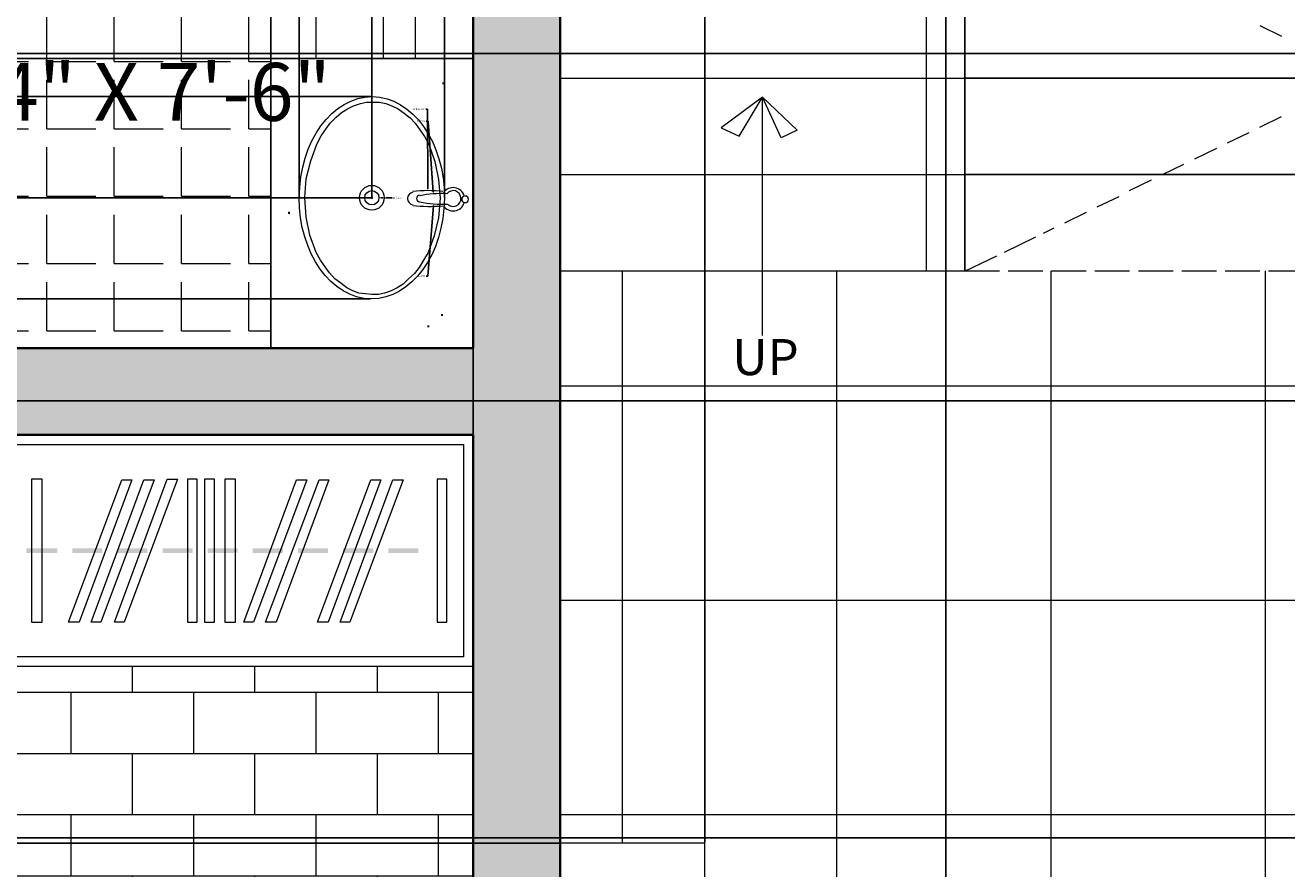
# Model space of a CAD drawing. Units: inches. Extents: x 6 to 575, y 34 to 566.
# Tile 10 of 21: x 151 to 282, y 387 to 474. Entities that reach past the tile are written whole.
import ezdxf

# ---------------------------------------------------------------- set-up
doc = ezdxf.new("R2010")
doc.units = ezdxf.units.IN
doc.linetypes.add('ACAD_ISO02W100', pattern=[15, 12, -3])
for name, color, linetype, lineweight in [('A-ANNO-DIMS', 2, 'Continuous', 18), ('A-ANNO-SYMB', 6, 'Continuous', 18), ('A-ANNO-TEXT', 6, 'Continuous', 18), ('A-AREA-IDEN', 6, 'Continuous', 20), ('A-FLOR-CASE', 2, 'Continuous', 18), ('A-FLOR-FIXT', 9, 'Continuous', 18), ('A-FLOR-PATT', 252, 'Continuous', 9), ('A-FLOR-STRS-OVHD', 1, 'ACAD_ISO02W100', 13), ('A-WALL-PATT', 251, 'Continuous', 9), ('STAIRS', 1, 'Continuous', 20), ('WALLS', 7, 'Continuous', 35)]:
    doc.layers.add(name, color=color, linetype=linetype, lineweight=lineweight)
doc.styles.add('PDF Arial Narrow', font='txt')
doc.styles.add('PDF Century Gothic', font='txt')
doc.styles.get("Standard").update_dxf_attribs({"font": 'arial.ttf'})
doc.dimstyles.get("Standard").update_dxf_attribs({"dimtxt": 0.18, "dimasz": 0.18, "dimexe": 0.18, "dimexo": 0.0625, "dimgap": 0.09, "dimtad": 0, "dimtih": 1, "dimtoh": 1, "dimdec": 4, "dimzin": 0, "dimdsep": 46, "dimtxsty": 'Standard', "dimcen": 0.09, "dimadec": 0, "dimazin": 0, "dimtfac": 1, "dimtdec": 4, "dimtofl": 0, "dimtmove": 0, "dimatfit": 3, "dimfxl": 1, "dimtolj": 1, "dimtzin": 0, "dimarcsym": 0})

# ---------------------------------------------------------------- blocks, each defined once
blk = doc.blocks.new('*D30')
at = {"layer": 'A-ANNO-DIMS', "color": 0, "lineweight": -2, "transparency": 16777216}
for p, q in [((32.6, 539.8), (6.65, 539.8)), ((6.83, 539.62), (6.83, 299.97)), ((6.83, 59.95), (6.83, 299.61)), ((197.62, 59.77), (6.65, 59.77))]:
    blk.add_line(p, q, dxfattribs=at)
at = {"layer": 'A-ANNO-DIMS', "color": 0, "transparency": 16777216}
for points in [[(6.8, 539.62), (6.86, 539.62), (6.83, 539.8)], [(6.8, 59.95), (6.86, 59.95), (6.83, 59.77)]]:
    blk.add_solid(points, dxfattribs=at)
at = {"layer": 'Defpoints', "color": 0, "transparency": 16777216}
for p in [(32.66, 539.8), (6.83, 59.77), (197.69, 59.77)]:
    blk.add_point(p, dxfattribs=at)
at = {"layer": 'A-ANNO-DIMS', "color": 0, "transparency": 16777216, "insert": (6.83, 299.79), "char_height": 0.18, "attachment_point": 5}
blk.add_mtext('\\A1;480', dxfattribs=at)
blk = doc.blocks.new('*D49')
at = {"layer": 'A-ANNO-DIMS', "color": 0, "lineweight": -2, "transparency": 16777216}
for p, q in [((206.66, 448.86), (206.66, 565.81)), ((206.84, 565.63), (227.18, 565.63)), ((248.45, 565.63), (228.11, 565.63)), ((248.63, 448.86), (248.63, 565.81))]:
    blk.add_line(p, q, dxfattribs=at)
at = {"layer": 'A-ANNO-DIMS', "color": 0, "transparency": 16777216}
for points in [[(206.84, 565.66), (206.84, 565.6), (206.66, 565.63)], [(248.45, 565.66), (248.45, 565.6), (248.63, 565.63)]]:
    blk.add_solid(points, dxfattribs=at)
at = {"layer": 'Defpoints', "color": 0, "transparency": 16777216}
for p in [(248.63, 565.63), (206.66, 448.8), (248.63, 448.8)]:
    blk.add_point(p, dxfattribs=at)
at = {"layer": 'A-ANNO-DIMS', "color": 0, "transparency": 16777216, "insert": (227.65, 565.63), "char_height": 0.18, "attachment_point": 5}
blk.add_mtext('\\A1;41.975', dxfattribs=at)
blk = doc.blocks.new('*D50')
at = {"layer": 'A-ANNO-DIMS', "color": 0, "lineweight": -2, "transparency": 16777216}
for p, q in [((248.7, 468.78), (574.68, 468.78)), ((574.5, 468.6), (574.5, 463.96)), ((574.5, 458.97), (574.5, 463.6)), ((248.7, 458.79), (574.68, 458.79))]:
    blk.add_line(p, q, dxfattribs=at)
at = {"layer": 'A-ANNO-DIMS', "color": 0, "transparency": 16777216}
for points in [[(574.47, 468.6), (574.53, 468.6), (574.5, 468.78)], [(574.47, 458.97), (574.53, 458.97), (574.5, 458.79)]]:
    blk.add_solid(points, dxfattribs=at)
at = {"layer": 'Defpoints', "color": 0, "transparency": 16777216}
for p in [(248.63, 468.78), (574.5, 468.78), (248.63, 458.79)]:
    blk.add_point(p, dxfattribs=at)
at = {"layer": 'A-ANNO-DIMS', "color": 0, "transparency": 16777216, "insert": (574.5, 463.78), "char_height": 0.18, "attachment_point": 5}
blk.add_mtext('\\A1;9.987', dxfattribs=at)
blk = doc.blocks.new('*D52')
at = {"layer": 'A-ANNO-DIMS', "color": 0, "lineweight": -2, "transparency": 16777216}
for p, q in [((437.62, 471.35), (6.65, 471.35)), ((6.83, 471.17), (6.83, 453.51)), ((6.83, 435.49), (6.83, 453.15)), ((437.62, 435.31), (6.65, 435.31))]:
    blk.add_line(p, q, dxfattribs=at)
at = {"layer": 'A-ANNO-DIMS', "color": 0, "transparency": 16777216}
for points in [[(6.8, 471.17), (6.86, 471.17), (6.83, 471.35)], [(6.8, 435.49), (6.86, 435.49), (6.83, 435.31)]]:
    blk.add_solid(points, dxfattribs=at)
at = {"layer": 'Defpoints', "color": 0, "transparency": 16777216}
for p in [(6.83, 471.35), (437.69, 471.35), (437.69, 435.31)]:
    blk.add_point(p, dxfattribs=at)
at = {"layer": 'A-ANNO-DIMS', "color": 0, "transparency": 16777216, "insert": (6.83, 453.33), "char_height": 0.18, "attachment_point": 5}
blk.add_mtext('\\A1;36.045', dxfattribs=at)
blk = doc.blocks.new('*D59')
at = {"layer": 'A-ANNO-DIMS', "color": 0, "lineweight": -2, "transparency": 16777216}
for p, q in [((206.66, 224.86), (206.66, 565.81)), ((206.84, 565.63), (226.44, 565.63)), ((246.48, 565.63), (226.88, 565.63)), ((246.66, 224.86), (246.66, 565.81))]:
    blk.add_line(p, q, dxfattribs=at)
at = {"layer": 'A-ANNO-DIMS', "color": 0, "transparency": 16777216}
for points in [[(206.84, 565.66), (206.84, 565.6), (206.66, 565.63)], [(246.48, 565.66), (246.48, 565.6), (246.66, 565.63)]]:
    blk.add_solid(points, dxfattribs=at)
at = {"layer": 'Defpoints', "color": 0, "transparency": 16777216}
for p in [(246.66, 565.63), (206.66, 224.8), (246.66, 224.8)]:
    blk.add_point(p, dxfattribs=at)
at = {"layer": 'A-ANNO-DIMS', "color": 0, "transparency": 16777216, "insert": (226.66, 565.63), "char_height": 0.18, "attachment_point": 5}
blk.add_mtext('\\A1;40', dxfattribs=at)
blk = doc.blocks.new('*D73')
at = {"layer": 'A-ANNO-DIMS', "color": 0, "lineweight": -2, "transparency": 16777216}
for p, q in [((248.63, 448.86), (248.63, 565.81)), ((248.81, 565.63), (285.25, 565.63)), ((322.48, 565.63), (286.04, 565.63)), ((322.66, 448.86), (322.66, 565.81))]:
    blk.add_line(p, q, dxfattribs=at)
at = {"layer": 'A-ANNO-DIMS', "color": 0, "transparency": 16777216}
for points in [[(248.81, 565.66), (248.81, 565.6), (248.63, 565.63)], [(322.48, 565.66), (322.48, 565.6), (322.66, 565.63)]]:
    blk.add_solid(points, dxfattribs=at)
at = {"layer": 'Defpoints', "color": 0, "transparency": 16777216}
for p in [(322.66, 565.63), (248.63, 448.8), (322.66, 448.8)]:
    blk.add_point(p, dxfattribs=at)
at = {"layer": 'A-ANNO-DIMS', "color": 0, "transparency": 16777216, "insert": (285.65, 565.63), "char_height": 0.18, "attachment_point": 5}
blk.add_mtext('\\A1;74.03', dxfattribs=at)
blk = doc.blocks.new('*D109')
at = {"layer": 'A-ANNO-DIMS', "color": 0, "lineweight": -2, "transparency": 16777216}
for p, q in [((112.85, 431.86), (112.85, 565.81)), ((113.03, 565.63), (154.93, 565.63)), ((197.48, 565.63), (155.58, 565.63)), ((197.66, 431.86), (197.66, 565.81))]:
    blk.add_line(p, q, dxfattribs=at)
at = {"layer": 'A-ANNO-DIMS', "color": 0, "transparency": 16777216}
for points in [[(113.03, 565.66), (113.03, 565.6), (112.85, 565.63)], [(197.48, 565.66), (197.48, 565.6), (197.66, 565.63)]]:
    blk.add_solid(points, dxfattribs=at)
at = {"layer": 'Defpoints', "color": 0, "transparency": 16777216}
for p in [(197.66, 565.63), (112.85, 431.8), (197.66, 431.8)]:
    blk.add_point(p, dxfattribs=at)
at = {"layer": 'A-ANNO-DIMS', "color": 0, "transparency": 16777216, "insert": (155.25, 565.63), "char_height": 0.18, "attachment_point": 5}
blk.add_mtext('\\A1;84.8', dxfattribs=at)
blk = doc.blocks.new('*D132')
at = {"layer": 'A-ANNO-DIMS', "color": 0, "lineweight": -2, "transparency": 16777216}
for p, q in [((288.54, 390), (6.65, 390)), ((6.83, 389.82), (6.83, 366.19)), ((6.83, 342.19), (6.83, 365.82)), ((288.54, 342.01), (6.65, 342.01))]:
    blk.add_line(p, q, dxfattribs=at)
at = {"layer": 'A-ANNO-DIMS', "color": 0, "transparency": 16777216}
for points in [[(6.8, 389.82), (6.86, 389.82), (6.83, 390)], [(6.8, 342.19), (6.86, 342.19), (6.83, 342.01)]]:
    blk.add_solid(points, dxfattribs=at)
at = {"layer": 'Defpoints', "color": 0, "transparency": 16777216}
for p in [(6.83, 390), (288.6, 390), (288.6, 342.01)]:
    blk.add_point(p, dxfattribs=at)
at = {"layer": 'A-ANNO-DIMS', "color": 0, "transparency": 16777216, "insert": (6.83, 366), "char_height": 0.18, "attachment_point": 5}
blk.add_mtext('\\A1;47.98', dxfattribs=at)
blk = doc.blocks.new('*D135')
at = {"layer": 'A-ANNO-DIMS', "color": 0, "lineweight": -2, "transparency": 16777216}
for p, q in [((206.68, 389.51), (206.68, 565.81)), ((206.86, 565.63), (213.79, 565.63)), ((221.48, 565.63), (214.56, 565.63)), ((221.66, 389.51), (221.66, 565.81))]:
    blk.add_line(p, q, dxfattribs=at)
at = {"layer": 'A-ANNO-DIMS', "color": 0, "transparency": 16777216}
for points in [[(206.86, 565.66), (206.86, 565.6), (206.68, 565.63)], [(221.48, 565.66), (221.48, 565.6), (221.66, 565.63)]]:
    blk.add_solid(points, dxfattribs=at)
at = {"layer": 'Defpoints', "color": 0, "transparency": 16777216}
for p in [(221.66, 565.63), (206.68, 389.45), (221.66, 389.45)]:
    blk.add_point(p, dxfattribs=at)
at = {"layer": 'A-ANNO-DIMS', "color": 0, "transparency": 16777216, "insert": (214.17, 565.63), "char_height": 0.18, "attachment_point": 5}
blk.add_mtext('\\A1;14.98', dxfattribs=at)
blk = doc.blocks.new('*D136')
at = {"layer": 'A-ANNO-DIMS', "color": 0, "lineweight": -2, "transparency": 16777216}
for p, q in [((206.62, 389.45), (6.65, 389.45)), ((6.83, 389.27), (6.83, 350.19)), ((6.83, 310.75), (6.83, 349.83)), ((206.62, 310.57), (6.65, 310.57))]:
    blk.add_line(p, q, dxfattribs=at)
at = {"layer": 'A-ANNO-DIMS', "color": 0, "transparency": 16777216}
for points in [[(6.8, 389.27), (6.86, 389.27), (6.83, 389.45)], [(6.8, 310.75), (6.86, 310.75), (6.83, 310.57)]]:
    blk.add_solid(points, dxfattribs=at)
at = {"layer": 'Defpoints', "color": 0, "transparency": 16777216}
for p in [(6.83, 389.45), (206.68, 389.45), (206.68, 310.57)]:
    blk.add_point(p, dxfattribs=at)
at = {"layer": 'A-ANNO-DIMS', "color": 0, "transparency": 16777216, "insert": (6.83, 350.01), "char_height": 0.18, "attachment_point": 5}
blk.add_mtext('\\A1;78.88', dxfattribs=at)
blk = doc.blocks.new('*D185')
at = {"layer": 'A-ANNO-DIMS', "color": 0, "lineweight": -2, "transparency": 16777216}
for p, q in [((176.67, 440.86), (176.67, 565.81)), ((176.85, 565.63), (186.7, 565.63)), ((197.48, 565.63), (187.63, 565.63)), ((197.66, 470.9), (197.66, 565.81))]:
    blk.add_line(p, q, dxfattribs=at)
at = {"layer": 'A-ANNO-DIMS', "color": 0, "transparency": 16777216}
for points in [[(176.85, 565.66), (176.85, 565.6), (176.67, 565.63)], [(197.48, 565.66), (197.48, 565.6), (197.66, 565.63)]]:
    blk.add_solid(points, dxfattribs=at)
at = {"layer": 'Defpoints', "color": 0, "transparency": 16777216}
for p in [(197.66, 565.63), (197.66, 470.84), (176.67, 440.8)]:
    blk.add_point(p, dxfattribs=at)
at = {"layer": 'A-ANNO-DIMS', "color": 0, "transparency": 16777216, "insert": (187.17, 565.63), "char_height": 0.18, "attachment_point": 5}
blk.add_mtext('\\A1;20.987', dxfattribs=at)
blk = doc.blocks.new('*D186')
at = {"layer": 'A-ANNO-DIMS', "color": 0, "lineweight": -2, "transparency": 16777216}
for p, q in [((197.6, 470.84), (6.65, 470.84)), ((6.83, 470.66), (6.83, 456)), ((6.83, 440.98), (6.83, 455.64)), ((176.61, 440.8), (6.65, 440.8))]:
    blk.add_line(p, q, dxfattribs=at)
at = {"layer": 'A-ANNO-DIMS', "color": 0, "transparency": 16777216}
for points in [[(6.8, 470.66), (6.86, 470.66), (6.83, 470.84)], [(6.8, 440.98), (6.86, 440.98), (6.83, 440.8)]]:
    blk.add_solid(points, dxfattribs=at)
at = {"layer": 'Defpoints', "color": 0, "transparency": 16777216}
for p in [(6.83, 470.84), (197.66, 470.84), (176.67, 440.8)]:
    blk.add_point(p, dxfattribs=at)
at = {"layer": 'A-ANNO-DIMS', "color": 0, "transparency": 16777216, "insert": (6.83, 455.82), "char_height": 0.18, "attachment_point": 5}
blk.add_mtext('\\A1;30.04', dxfattribs=at)
blk = doc.blocks.new('*D187')
at = {"layer": 'A-ANNO-DIMS', "color": 0, "lineweight": -2, "transparency": 16777216}
for p, q in [((179.61, 456.49), (179.61, 565.81)), ((179.79, 565.63), (186.69, 565.63)), ((194.49, 565.63), (187.6, 565.63)), ((194.67, 456.4), (194.67, 565.81))]:
    blk.add_line(p, q, dxfattribs=at)
at = {"layer": 'A-ANNO-DIMS', "color": 0, "transparency": 16777216}
for points in [[(179.79, 565.66), (179.79, 565.6), (179.61, 565.63)], [(194.49, 565.66), (194.49, 565.6), (194.67, 565.63)]]:
    blk.add_solid(points, dxfattribs=at)
at = {"layer": 'Defpoints', "color": 0, "transparency": 16777216}
for p in [(194.67, 565.63), (179.61, 456.43), (194.67, 456.34)]:
    blk.add_point(p, dxfattribs=at)
at = {"layer": 'A-ANNO-DIMS', "color": 0, "transparency": 16777216, "insert": (187.14, 565.63), "char_height": 0.18, "attachment_point": 5}
blk.add_mtext('\\A1;15.058', dxfattribs=at)
blk = doc.blocks.new('*D188')
at = {"layer": 'A-ANNO-DIMS', "color": 0, "lineweight": -2, "transparency": 16777216}
for p, q in [((187.14, 466.88), (6.65, 466.88)), ((6.83, 466.7), (6.83, 456.56)), ((6.83, 446.07), (6.83, 456.2)), ((187.02, 445.89), (6.65, 445.89))]:
    blk.add_line(p, q, dxfattribs=at)
at = {"layer": 'A-ANNO-DIMS', "color": 0, "transparency": 16777216}
for points in [[(6.8, 466.7), (6.86, 466.7), (6.83, 466.88)], [(6.8, 446.07), (6.86, 446.07), (6.83, 445.89)]]:
    blk.add_solid(points, dxfattribs=at)
at = {"layer": 'Defpoints', "color": 0, "transparency": 16777216}
for p in [(6.83, 466.88), (187.2, 466.88), (187.08, 445.89)]:
    blk.add_point(p, dxfattribs=at)
at = {"layer": 'A-ANNO-DIMS', "color": 0, "transparency": 16777216, "insert": (6.83, 456.38), "char_height": 0.18, "attachment_point": 5}
blk.add_mtext('\\A1;20.987', dxfattribs=at)
blk = doc.blocks.new('*D189')
at = {"layer": 'A-ANNO-DIMS', "color": 0, "lineweight": -2, "transparency": 16777216}
for p, q in [((187.08, 456.38), (6.65, 456.38)), ((6.83, 456.2), (6.83, 448.77)), ((6.83, 440.98), (6.83, 448.41)), ((197.6, 440.8), (6.65, 440.8))]:
    blk.add_line(p, q, dxfattribs=at)
at = {"layer": 'A-ANNO-DIMS', "color": 0, "transparency": 16777216}
for points in [[(6.8, 456.2), (6.86, 456.2), (6.83, 456.38)], [(6.8, 440.98), (6.86, 440.98), (6.83, 440.8)]]:
    blk.add_solid(points, dxfattribs=at)
at = {"layer": 'Defpoints', "color": 0, "transparency": 16777216}
for p in [(6.83, 456.38), (187.14, 456.38), (197.66, 440.8)]:
    blk.add_point(p, dxfattribs=at)
at = {"layer": 'A-ANNO-DIMS', "color": 0, "transparency": 16777216, "insert": (6.83, 448.59), "char_height": 0.18, "attachment_point": 5}
blk.add_mtext('\\A1;15.582', dxfattribs=at)
blk = doc.blocks.new('*D190')
at = {"layer": 'A-ANNO-DIMS', "color": 0, "lineweight": -2, "transparency": 16777216}
for p, q in [((187.14, 456.45), (187.14, 565.81)), ((187.32, 565.63), (191.95, 565.63)), ((197.48, 565.63), (192.86, 565.63)), ((197.66, 440.86), (197.66, 565.81))]:
    blk.add_line(p, q, dxfattribs=at)
at = {"layer": 'A-ANNO-DIMS', "color": 0, "transparency": 16777216}
for points in [[(187.32, 565.66), (187.32, 565.6), (187.14, 565.63)], [(197.48, 565.66), (197.48, 565.6), (197.66, 565.63)]]:
    blk.add_solid(points, dxfattribs=at)
at = {"layer": 'Defpoints', "color": 0, "transparency": 16777216}
for p in [(187.14, 565.63), (187.14, 456.38), (197.66, 440.8)]:
    blk.add_point(p, dxfattribs=at)
at = {"layer": 'A-ANNO-DIMS', "color": 0, "transparency": 16777216, "insert": (192.4, 565.63), "char_height": 0.18, "attachment_point": 5}
blk.add_mtext('\\A1;10.516', dxfattribs=at)
blk = doc.blocks.new('*D226')
at = {"layer": 'A-ANNO-DIMS', "color": 0, "lineweight": -2, "transparency": 16777216}
for p, q in [((192.35, 536.37), (187.21, 505.96)), ((192.53, 536.37), (192.35, 536.37)), ((178.47, 454.82), (178.65, 454.82)), ((178.56, 454.73), (178.56, 454.91))]:
    blk.add_line(p, q, dxfattribs=at)
at = {"layer": 'A-ANNO-DIMS', "color": 0, "transparency": 16777216}
blk.add_solid([(187.18, 505.97), (187.24, 505.96), (187.18, 505.79)], dxfattribs=at)
at = {"layer": 'Defpoints', "color": 0, "transparency": 16777216}
for p in [(187.18, 505.79), (178.56, 454.82)]:
    blk.add_point(p, dxfattribs=at)
at = {"layer": 'A-ANNO-DIMS', "color": 0, "transparency": 16777216, "insert": (193.21, 536.37), "char_height": 0.18, "attachment_point": 5}
blk.add_mtext('\\A1;2X R51.69', dxfattribs=at)
blk = doc.blocks.new('*D231')
at = {"layer": 'A-ANNO-DIMS', "color": 0, "lineweight": -2, "transparency": 16777216}
for p, q in [((192.75, 465.57), (192.93, 465.57)), ((192.93, 465.57), (192.95, 457.3)), ((192.9, 443.04), (193.08, 443.04)), ((192.99, 442.95), (192.99, 443.13))]:
    blk.add_line(p, q, dxfattribs=at)
at = {"layer": 'A-ANNO-DIMS', "color": 0, "transparency": 16777216}
blk.add_solid([(192.98, 457.3), (192.92, 457.3), (192.95, 457.12)], dxfattribs=at)
at = {"layer": 'Defpoints', "color": 0, "transparency": 16777216}
for p in [(192.95, 457.12), (192.99, 443.04)]:
    blk.add_point(p, dxfattribs=at)
at = {"layer": 'A-ANNO-DIMS', "color": 0, "transparency": 16777216, "insert": (192, 465.57), "char_height": 0.18, "attachment_point": 5}
blk.add_mtext('\\A1;4X R14.083', dxfattribs=at)
blk = doc.blocks.new('*D232')
at = {"layer": 'A-ANNO-DIMS', "color": 0, "lineweight": -2, "transparency": 16777216}
for p, q in [((192.79, 464.32), (192.97, 464.32)), ((192.97, 464.32), (193.5, 456.96)), ((194.33, 444.22), (194.51, 444.22)), ((194.42, 444.13), (194.42, 444.31))]:
    blk.add_line(p, q, dxfattribs=at)
at = {"layer": 'A-ANNO-DIMS', "color": 0, "transparency": 16777216}
blk.add_solid([(193.53, 456.96), (193.47, 456.96), (193.51, 456.78)], dxfattribs=at)
at = {"layer": 'Defpoints', "color": 0, "transparency": 16777216}
for p in [(193.51, 456.78), (194.42, 444.22)]:
    blk.add_point(p, dxfattribs=at)
at = {"layer": 'A-ANNO-DIMS', "color": 0, "transparency": 16777216, "insert": (192.24, 464.32), "char_height": 0.18, "attachment_point": 5}
blk.add_mtext('\\A1;R12.594', dxfattribs=at)
blk = doc.blocks.new('*D234')
at = {"layer": 'A-ANNO-DIMS', "color": 0, "lineweight": -2, "transparency": 16777216}
for p, q in [((194.46, 468.24), (194.64, 468.24)), ((194.55, 468.15), (194.55, 468.33)), ((192.95, 448.27), (193.54, 455.58)), ((192.77, 448.27), (192.95, 448.27))]:
    blk.add_line(p, q, dxfattribs=at)
at = {"layer": 'A-ANNO-DIMS', "color": 0, "transparency": 16777216}
blk.add_solid([(193.51, 455.58), (193.57, 455.58), (193.55, 455.76)], dxfattribs=at)
at = {"layer": 'Defpoints', "color": 0, "transparency": 16777216}
for p in [(194.55, 468.24), (193.55, 455.76)]:
    blk.add_point(p, dxfattribs=at)
at = {"layer": 'A-ANNO-DIMS', "color": 0, "transparency": 16777216, "insert": (192.29, 448.27), "char_height": 0.18, "attachment_point": 5}
blk.add_mtext('\\A1;R12.52', dxfattribs=at)
blk = doc.blocks.new('*D252')
at = {"layer": 'A-ANNO-DIMS', "color": 0, "lineweight": -2, "transparency": 16777216}
for p, q in [((187.05, 456.38), (187.23, 456.38)), ((187.14, 456.29), (187.14, 456.47)), ((189.2, 456.39), (188.61, 456.39))]:
    blk.add_line(p, q, dxfattribs=at)
at = {"layer": 'A-ANNO-DIMS', "color": 0, "transparency": 16777216}
blk.add_solid([(188.61, 456.42), (188.61, 456.36), (188.43, 456.39)], dxfattribs=at)
at = {"layer": 'Defpoints', "color": 0, "transparency": 16777216}
for p in [(185.85, 456.38), (188.43, 456.39)]:
    blk.add_point(p, dxfattribs=at)
at = {"layer": 'A-ANNO-DIMS', "color": 0, "transparency": 16777216, "insert": (189.81, 456.39), "char_height": 0.18, "attachment_point": 5}
blk.add_mtext('\\A1;2X ∅2.57', dxfattribs=at)
blk = doc.blocks.new('*D253')
at = {"layer": 'A-ANNO-DIMS', "color": 0, "lineweight": -2, "transparency": 16777216}
for p, q in [((187.05, 456.38), (187.23, 456.38)), ((187.14, 456.29), (187.14, 456.47)), ((188.33, 456.39), (188.06, 456.39))]:
    blk.add_line(p, q, dxfattribs=at)
at = {"layer": 'A-ANNO-DIMS', "color": 0, "transparency": 16777216}
blk.add_solid([(188.06, 456.42), (188.06, 456.36), (187.88, 456.39)], dxfattribs=at)
at = {"layer": 'Defpoints', "color": 0, "transparency": 16777216}
for p in [(186.4, 456.38), (187.88, 456.39)]:
    blk.add_point(p, dxfattribs=at)
at = {"layer": 'A-ANNO-DIMS', "color": 0, "transparency": 16777216, "insert": (188.94, 456.39), "char_height": 0.18, "attachment_point": 5}
blk.add_mtext('\\A1;2X ∅1.48', dxfattribs=at)

msp = doc.modelspace()

# ---------------------------------------------------------------- hatches: boundary and pattern name
at = {"layer": 'A-FLOR-PATT'}
h = msp.add_hatch(dxfattribs=at)
h.set_pattern_fill('ANGLE', color=256)
h.set_pattern_definition([(0, (-98.035, 170.1465), (0, 6.985), [5.08, -1.905]), (90, (-98.035, 170.1465), (-6.985, 4e-16), [5.08, -1.905])])
edge = h.paths.add_edge_path()
edge.add_line((191.6511, 494.1664), (190.4028, 493.9036))
edge.add_line((190.4028, 493.9036), (189.6226, 493.6983))
edge.add_line((189.6226, 493.6983), (188.2183, 493.3862))
edge.add_line((188.2183, 493.3862), (187.2685, 493.2437))
edge.add_line((187.2685, 493.2437), (187.204, 493.2302))
edge.add_line((187.204, 493.2302), (187.0709, 493.2141))
edge.add_line((187.0709, 493.2141), (185.0975, 492.9181))
edge.add_line((185.0975, 492.9181), (185.0904, 492.9751))
edge.add_line((185.0904, 492.9751), (183.6001, 492.7952))
edge.add_line((183.6001, 492.7952), (183.5371, 492.7621))
edge.add_line((183.5371, 492.7621), (181.5041, 492.4232))
edge.add_spline(control_points=[(181.5178, 492.4356), (181.2536, 492.4138), (180.9898, 492.4), (180.727, 492.3941)], knot_values=[2.92921633, 2.92921633, 2.92921633, 2.92921633, 3, 3, 3, 3], degree=3, periodic=0)
edge.add_line((180.727, 492.3941), (180.4943, 492.372))
edge.add_line((180.4943, 492.372), (180.175, 492.3932))
edge.add_spline(control_points=[(180.175, 492.3932), (179.0187, 492.4156), (177.8901, 492.5895), (176.8377, 492.8977)], knot_values=[2.56593531, 2.56593531, 2.56593531, 2.56593531, 2.87949124, 2.87949124, 2.87949124, 2.87949124], degree=3, periodic=0)
edge.add_line((176.8377, 492.8977), (176.5264, 492.9696))
edge.add_spline(control_points=[(176.656, 492.9525), (176.2658, 493.0735), (175.8866, 493.2132), (175.521, 493.3707)], knot_values=[2.43053183, 2.43053183, 2.43053183, 2.43053183, 2.54781219, 2.54781219, 2.54781219, 2.54781219], degree=3, periodic=0)
edge.add_line((175.521, 493.3707), (175.267, 493.4642))
edge.add_line((175.267, 493.4642), (175.098, 493.5637))
edge.add_spline(control_points=[(175.098, 493.5637), (173.9351, 494.1251), (172.9292, 494.8734), (172.1696, 495.7766)], knot_values=[2, 2, 2, 2, 2.38461715, 2.38461715, 2.38461715, 2.38461715], degree=3, periodic=0)
edge.add_line((172.9656, 494.9581), (172.8363, 495.1004))
edge.add_spline(control_points=[(175.098, 493.5637), (173.9351, 494.1251), (172.9292, 494.8734), (172.1696, 495.7766)], knot_values=[2, 2, 2, 2, 2.38461715, 2.38461715, 2.38461715, 2.38461715], degree=3, periodic=0)
edge.add_line((171.9925, 495.9563), (171.8762, 496.1888))
edge.add_spline(control_points=[(172.1696, 495.7766), (170.1947, 498.1251), (170.2393, 501.0999), (172.2842, 503.4158)], knot_values=[1, 1, 1, 1, 2, 2, 2, 2], degree=3, periodic=0)
edge.add_line((170.6556, 499.1388), (170.6881, 499.323))
edge.add_spline(control_points=[(172.1696, 495.7766), (170.1947, 498.1251), (170.2393, 501.0999), (172.2842, 503.4158)], knot_values=[1, 1, 1, 1, 2, 2, 2, 2], degree=3, periodic=0)
edge.add_spline(control_points=[(172.2842, 503.4158), (174.3291, 505.7317), (178.0076, 506.9734), (181.7304, 506.6045)], knot_values=[0, 0, 0, 0, 1, 1, 1, 1], degree=3, periodic=0)
edge.add_line((174.0548, 504.9343), (174.2554, 505.022))
edge.add_spline(control_points=[(172.2842, 503.4158), (174.3291, 505.7317), (178.0076, 506.9734), (181.7304, 506.6045)], knot_values=[0, 0, 0, 0, 1, 1, 1, 1], degree=3, periodic=0)
edge.add_line((178.4031, 506.5313), (178.1947, 506.4718))
edge.add_spline(control_points=[(172.2842, 503.4158), (174.3291, 505.7317), (178.0076, 506.9734), (181.7304, 506.6045)], knot_values=[0, 0, 0, 0, 1, 1, 1, 1], degree=3, periodic=0)
edge.add_line((181.5796, 506.6123), (181.6459, 506.5957))
edge.add_arc((179.34, 495.0824), 11.742, 73.636084, 78.674278, ccw=False)
edge.add_arc((178.5598, 454.8227), 51.688, 83.52982, 85.463383, ccw=False)
edge.add_line((184.3843, 506.1814), (184.5513, 506.1814))
edge.add_line((184.5513, 506.1814), (184.7887, 506.134))
edge.add_arc((178.5598, 454.8227), 51.688, 75.328548, 83.07845, ccw=False)
edge.add_line((191.6511, 504.8253), (191.6511, 530.801))
edge.add_line((191.6511, 530.801), (184.6586, 530.801))
edge.add_line((184.6586, 530.801), (160.6586, 530.801))
edge.add_line((160.6586, 530.801), (157.8686, 530.801))
edge.add_line((157.8686, 530.801), (157.8686, 488.7831))
edge.add_line((157.8686, 488.7831), (121.6586, 488.7831))
edge.add_line((121.6586, 488.7831), (121.6586, 474.801))
edge.add_line((121.6586, 474.801), (120.6068, 474.801))
edge.add_line((120.6068, 474.801), (120.6068, 474.0666))
edge.add_arc((120.0902, 447.538), 26.5336, 62.388015, 88.884314, ccw=False)
edge.add_line((132.388, 471.0496), (132.3995, 471.0696))
edge.add_line((132.3995, 471.0696), (133.357, 470.5168))
edge.add_line((133.357, 470.5168), (120.0902, 447.538))
edge.add_line((120.0902, 447.538), (120.6068, 447.538))
edge.add_line((120.6068, 447.538), (121.6586, 446.801))
edge.add_line((121.6586, 446.801), (121.6586, 440.801))
edge.add_line((121.6586, 440.801), (176.6714, 440.801))
edge.add_line((176.6714, 440.801), (176.6714, 470.8385))
edge.add_line((176.6714, 470.8385), (191.6511, 470.8385))
edge.add_line((191.6511, 470.8385), (191.6511, 494.1664))
h = msp.add_hatch(dxfattribs=at)
h.set_pattern_fill('BRICK', color=256)
h.set_pattern_definition([(0, (-98.035, 170.1465), (0, 6.35), []), (90, (-98.035, 170.147), (-12.7, 8e-16), [6.35, -6.35]), (90, (-91.685, 170.147), (-12.7, 8e-16), [-6.35, 6.35])])
h.paths.add_polyline_path([(180.8711, 269.7588), (182.4439, 270.6668), (182.4628, 270.6341, -0.11619827), (201.8275, 275.5902), (201.8275, 276.801), (197.6586, 276.801), (197.6586, 293.1641), (182.6401, 293.1641), (182.6401, 348.324), (197.6586, 348.324), (197.6586, 407.7709), (112.8513, 407.7709), (112.8513, 431.801), (111.6586, 431.801), (111.6586, 440.801), (117.6586, 440.801), (117.6586, 446.801), (117.6586, 448.2751), (117.6586, 473.3269), (117.6586, 474.801), (117.6586, 515.5941), (100.2533, 515.5941, -1), (83.0548, 515.5941), (65.6494, 515.5941), (65.6494, 440.801), (82.8918, 440.801), (82.8918, 431.801), (82.8918, 407.7709), (41.6586, 407.7709), (41.6586, 379.0637), (62.6459, 379.0637), (62.6459, 358.0764), (122.565, 358.0764), (122.565, 286.0643), (62.6459, 286.0643), (62.6459, 265.077), (41.6586, 265.077), (41.6586, 224.801), (41.6586, 212.801), (71.6586, 212.801), (167.6586, 212.801), (197.6586, 212.801), (197.6586, 230.801), (201.8157, 230.801), (201.8157, 233.4817)])
h.paths.add_polyline_path([(133.3414, 245.1275), (133.3317, 245.1352), (133.3317, 245.104)], flags=16)
h.paths.add_polyline_path([(133.3317, 222.1662), (85.3496, 222.1662), (85.3496, 243.7443, -0.50090726), (87.1831, 246.1963), (107.4292, 246.1963), (111.2522, 246.1963), (131.4202, 246.1963, -0.41421356), (133.3317, 244.2848)], flags=16)
h.paths.add_polyline_path([(72.7105, 244.4018), (72.7105, 220.3718), (48.6804, 220.3718), (48.6804, 244.4018)], flags=16)
h.paths.add_polyline_path([(71.7466, 237.8955, -1), (59.8096, 237.8955, -1)], flags=0)
h = msp.add_hatch(dxfattribs=at)
h.set_pattern_fill('NET', color=256, scale=7)
h.set_pattern_definition([(0, (-98.035, 170.147), (0, 22.225), []), (90, (-98.035, 170.147), (-22.225, 1e-15), [])])
h.paths.add_polyline_path([(368.183, 395.6385, -0.88370529), (374.2533, 394.8861), (374.6586, 448.801), (354.6586, 448.801), (354.6586, 448.7938), (353.1847, 448.7938), (326.6586, 448.801), (322.6586, 448.801), (248.6332, 448.8024), (206.6586, 448.8024), (206.6586, 389.449), (221.6622, 389.449), (221.6622, 310.5712), (206.6586, 310.5712), (206.6586, 276.801), (206.6704, 276.801), (206.6704, 274.3795), (206.6586, 224.801), (246.6586, 224.801), (264.6586, 224.801), (265.6986, 224.801), (265.6986, 249.081), (267.5186, 249.081), (267.5186, 249.0145, -0.38515288), (290.6494, 224.801), (290.6679, 224.801, -0.38515288), (313.7986, 249.0145), (313.7986, 249.081), (315.6186, 249.081), (315.6186, 224.801), (316.6586, 224.801), (334.6586, 224.801), (374.6586, 224.801), (374.6586, 278.801), (374.1753, 318.8919, -0.45530286), (370.7577, 315.9168), (370.6643, 313.8205, -0.41421356), (368.7528, 311.909), (368.8072, 311.8975), (368.7528, 311.909, 0.41421356), (370.6643, 313.8205), (370.7632, 315.9161, -0.34634601), (368.183, 318.5897)])
h.paths.add_polyline_path([(288.603, 342.0131), (288.603, 389.9952), (318.6406, 389.9952), (318.6406, 342.0131)], flags=16)
h.paths.add_polyline_path([(289.6173, 343.0274), (289.6173, 389.059), (317.6263, 389.059), (317.6263, 343.0274)], flags=0)
h.paths.add_polyline_path([(295.4867, 311.7535, 0.06538163), (295.1241, 312.0945), (295.0006, 312.1316)], flags=16)
h.paths.add_polyline_path([(328.4931, 284.9911, 0.41421356), (330.4045, 286.9026), (330.4215, 286.8532), (330.4045, 286.9026, -0.41421356), (328.4931, 284.9911), (328.549, 284.9808)], flags=16)
h.paths.add_polyline_path([(344.7771, 305.2659), (368.8072, 305.2659), (368.8072, 281.2358), (344.7771, 281.2358)], flags=16)
h.paths.add_polyline_path([(368.183, 288.1406, -1), (356.246, 288.1406, -1)], flags=0)
h.paths.add_polyline_path([(347.9759, 404.6629), (347.9759, 428.6929), (372.006, 428.6929), (372.006, 404.6629)], flags=16)
h.paths.add_polyline_path([(359.4448, 421.7882, -1), (371.3818, 421.7882, -1)], flags=0)
at = {"layer": 'A-WALL-PATT'}
h = msp.add_hatch(color=256, dxfattribs=at)
h.dxf.hatch_style = 1
h.paths.add_polyline_path([(160.6586, 539.801), (32.6586, 539.801), (32.6586, 272.801), (41.6586, 272.801), (41.6586, 286.0643), (41.6586, 358.0764), (41.6586, 379.0637), (41.6586, 407.7709), (41.6194, 407.7709), (41.6194, 431.801), (82.8918, 431.801), (82.8918, 440.801), (65.6494, 440.801), (65.6494, 440.7732), (41.6194, 440.7732), (41.6194, 515.5941), (41.6586, 530.801), (117.6586, 530.801), (117.6586, 474.801), (120.6068, 474.801), (121.6586, 474.801), (121.6586, 530.801), (137.4275, 530.801), (137.4275, 530.8356), (141.2505, 530.8356), (160.6586, 530.801)])
h.paths.add_polyline_path([(71.6586, 212.801), (41.6586, 212.801), (41.6586, 224.801), (32.6586, 224.801), (32.6586, 203.801), (71.6586, 203.801)])
h.paths.add_polyline_path([(206.6586, 215.801), (246.6586, 215.801), (246.6586, 224.801), (206.6586, 224.801), (206.6586, 230.801), (201.8157, 230.801), (197.6586, 230.801), (197.6586, 212.801), (167.6586, 212.801), (167.6586, 203.801), (206.6586, 203.801)])
h.paths.add_polyline_path([(383.6586, 224.801), (334.6586, 224.801), (334.6586, 215.801), (374.6586, 215.801), (374.6586, 203.801), (384.0753, 203.801), (407.6586, 203.801), (407.6586, 212.801), (383.6586, 212.801)])
h.paths.add_polyline_path([(548.6586, 270.801), (539.6586, 270.801), (539.6586, 212.801), (515.6586, 212.801), (515.6586, 203.801), (548.6586, 203.801)])
h.paths.add_polyline_path([(548.6586, 412.801), (545.7108, 412.801), (539.6586, 412.801), (539.6586, 382.801), (433.708, 382.801), (433.708, 378.801), (539.6586, 378.801), (539.6586, 366.801), (548.6586, 366.801)])
h.paths.add_polyline_path([(548.6586, 539.801), (455.9436, 539.801), (455.9436, 530.801), (539.6586, 530.801), (539.6586, 440.801), (548.6586, 440.801)])
h.paths.add_polyline_path([(407.9436, 539.801), (362.6586, 539.801), (362.6586, 530.801), (374.6586, 530.801), (374.6586, 452.801), (354.6586, 452.801), (354.6586, 448.801), (374.6586, 448.801), (374.6586, 278.801), (383.6586, 278.801), (383.6586, 530.801), (407.9436, 530.801)])
h.paths.add_polyline_path([(338.6586, 539.801), (320.6586, 539.801), (320.6586, 530.801), (322.6586, 530.801), (322.6586, 448.801), (326.6586, 448.801), (326.6586, 530.801), (338.6586, 530.801)])
h.paths.add_polyline_path([(272.6586, 539.801), (184.6586, 539.801), (184.6586, 530.801), (197.6586, 530.801), (197.6586, 440.801), (176.6714, 440.801), (121.6586, 440.801), (121.6586, 446.801), (117.6586, 446.801), (117.6586, 440.801), (111.6586, 440.801), (111.6586, 431.801), (197.6586, 431.801), (197.6586, 407.7709), (197.6586, 276.801), (206.6586, 276.801), (206.6586, 530.801), (272.6586, 530.801)])

# ---------------------------------------------------------------- linework, layer by layer
at = {"layer": 'A-ANNO-SYMB'}
msp.add_lwpolyline([(227.6459, 442.0927), (227.6459, 466.8249), (223.3548, 463.6261), (225.2273, 462.7679), (227.6459, 466.8249), (231.2348, 463.392), (229.5964, 462.6118), (227.6459, 466.8249)], dxfattribs=at)
at = {"layer": 'A-FLOR-CASE'}
msp.add_lwpolyline([(191.6511, 530.8356), (191.6511, 470.8385)], dxfattribs=at)
for points in [[(197.6586, 440.801), (176.6714, 440.801), (176.6714, 470.8385), (197.6586, 470.8385)], [(197.6586, 407.7709), (112.8513, 407.7709), (112.8513, 431.801), (197.6586, 431.801)], [(196.6444, 408.7852), (113.8656, 408.7852), (113.8656, 430.7867), (196.6444, 430.7867)], [(152.9534, 412.3741), (152.9534, 427.1978), (151.8611, 427.1978), (151.8611, 412.3741)], [(155.6841, 412.3741), (161.2235, 427.1198), (162.2377, 427.1198), (156.7764, 412.3741)], [(158.0247, 412.3741), (163.486, 427.1198), (164.5783, 427.1198), (159.0389, 412.3741)], [(160.4433, 412.3741), (165.9047, 427.1978), (166.9969, 427.1978), (161.4575, 412.3741)], [(169.0254, 412.3741), (169.0254, 427.1978), (168.0112, 427.1978), (168.0112, 412.3741)], [(170.8199, 412.3741), (170.8199, 427.1978), (169.8056, 427.1978), (169.8056, 412.3741)], [(173.0044, 412.3741), (173.0044, 427.1978), (171.9122, 427.1978), (171.9122, 412.3741)], [(173.8627, 412.3741), (179.324, 427.1198), (180.4163, 427.1198), (174.8769, 412.3741)], [(176.1252, 412.3741), (181.6646, 427.1198), (182.6789, 427.1198), (177.2175, 412.3741)], [(181.5086, 412.3741), (187.048, 427.1198), (188.0622, 427.1198), (182.6009, 412.3741)], [(183.8492, 412.3741), (189.3105, 427.1198), (190.4028, 427.1198), (184.8634, 412.3741)], [(194.928, 412.3741), (194.928, 427.1978), (193.9137, 427.1978), (193.9137, 412.3741)], [(206.6824, 389.449), (206.6824, 310.5712), (221.6622, 310.5712), (221.6622, 389.449)]]:
    msp.add_lwpolyline(points, close=True, dxfattribs=at)
at = {"layer": 'A-FLOR-CASE', "transparency": 33554559}
for points in [[(151.315, 420.02), (151.315, 419.5519), (154.5138, 420.02)], [(151.315, 419.5519), (154.5138, 420.02), (154.5138, 419.5519)], [(156.0742, 420.02), (156.0742, 419.5519), (159.195, 420.02)], [(156.0742, 419.5519), (159.195, 420.02), (159.195, 419.5519)], [(160.7554, 420.02), (160.7554, 419.5519), (163.8761, 420.02)], [(160.7554, 419.5519), (163.8761, 420.02), (163.8761, 419.5519)], [(165.4365, 420.02), (165.4365, 419.5519), (168.5573, 420.02)], [(165.4365, 419.5519), (168.5573, 420.02), (168.5573, 419.5519)], [(170.1177, 420.02), (170.1177, 419.5519), (173.2385, 420.02)], [(170.1177, 419.5519), (173.2385, 420.02), (173.2385, 419.5519)], [(174.7989, 420.02), (174.7989, 419.5519), (177.9197, 420.02)], [(174.7989, 419.5519), (177.9197, 420.02), (177.9197, 419.5519)], [(179.4801, 420.02), (179.4801, 419.5519), (182.6009, 420.02)], [(179.4801, 419.5519), (182.6009, 420.02), (182.6009, 419.5519)], [(184.1612, 420.02), (184.1612, 419.5519), (187.282, 420.02)], [(184.1612, 419.5519), (187.282, 420.02), (187.282, 419.5519)], [(188.8424, 420.02), (188.8424, 419.5519), (191.9632, 420.02)], [(188.8424, 419.5519), (191.9632, 420.02), (191.9632, 419.5519)]]:
    msp.add_solid(points, dxfattribs=at)
at = {"layer": 'A-FLOR-FIXT'}
msp.add_lwpolyline([(187.282, 466.3134), (187.9062, 466.3134), (188.6084, 466.1574), (189.2325, 465.9233), (189.8567, 465.6112), (190.4808, 465.1431), (191.105, 464.675), (191.6511, 464.1289), (192.1193, 463.4267), (192.5874, 462.7245), (193.0555, 461.9443), (193.6796, 460.1499), (194.0697, 458.2774), (194.2258, 456.3269), (194.0697, 454.2984), (193.6016, 452.4259), (192.9775, 450.7095), (192.5093, 449.9293), (192.0412, 449.1491), (191.5731, 448.5249), (190.949, 447.9788), (190.4028, 447.4327), (189.7787, 447.0426), (189.1545, 446.7305), (188.4523, 446.4964), (187.8282, 446.3404), (187.126, 446.3404), (186.5018, 446.4184), (185.7997, 446.4964), (185.1755, 446.7305), (184.5513, 447.0426), (183.9272, 447.5107), (183.303, 447.9788), (182.7569, 448.6029), (182.2888, 449.2271), (181.8207, 449.9293), (181.3525, 450.7095), (180.7284, 452.5039), (180.3383, 454.3764), (180.1822, 456.4049), (180.3383, 458.3554), (180.8064, 460.2279), (181.4306, 461.9443), (181.8987, 462.8025), (182.3668, 463.5047), (182.8349, 464.1289), (183.4591, 464.753), (184.0052, 465.2211), (184.6294, 465.6112), (185.2535, 465.9233), (185.9557, 466.1574), (186.5799, 466.3134)], close=True, dxfattribs=at)
msp.add_lwpolyline([(192.1279, 455.9576, 0.05744374), (194.9861, 455.7292, 2.66597622), (194.9195, 456.8047, 0.05597701), (192.1158, 456.6021)], format="xyb", dxfattribs=at)
for points in [[(196.9565, 456.5609), (196.8004, 456.5609)], [(196.9565, 455.8588), (196.8004, 455.8588)]]:
    msp.add_lwpolyline(points, dxfattribs=at)
for radius in [1.2873, 0.7412]:
    msp.add_circle((187.1423, 456.3831), radius, dxfattribs=at)
for centre, radius, start, end in [((191.5116, 456.3051), 0.6632, 99.915126, 259.414585), ((192.994, 443.0412), 14.0828, 83.798166, 96.553252), ((192.1358, 456.3051), 0.3511, 96.82233, 262.507381), ((195.5687, 456.227), 1.2093, 16.627786, 145.107366), ((193.15, 469.569), 14.0828, 262.776459, 275.531545), ((195.5687, 456.227), 1.2093, 214.222345, 342.701926), ((196.8171, 456.227), 0.3511, 99.909595, 259.420117), ((196.8171, 456.227), 0.3511, 279.909595, 79.420117)]:
    msp.add_arc(centre, radius, start, end, dxfattribs=at)
msp.add_open_spline([(179.6134, 456.4271), (179.5795, 450.6316), (182.9228, 445.9138), (187.0809, 445.8894), (191.239, 445.8651), (194.6373, 450.5436), (194.6712, 456.339), (194.7051, 462.1345), (191.3617, 466.8524), (187.2036, 466.8767), (183.0456, 466.901), (179.6473, 462.2226), (179.6134, 456.4271)], degree=3, knots=[0, 0, 0, 0, 1, 1, 1, 2, 2, 2, 3, 3, 3, 4, 4, 4, 4], dxfattribs=at)
at = {"layer": 'A-FLOR-STRS-OVHD', "ltscale": 0.3}
msp.add_line((248.6332, 448.8024), (322.6586, 448.8024), dxfattribs=at)
at = {"layer": 'A-FLOR-STRS-OVHD'}
for points in [[(279.2169, 474.2368), (281.4795, 473.1445)], [(279.2169, 463.7041), (281.4795, 464.7964)], [(275.8621, 462.0657), (278.1246, 463.158)], [(272.5072, 460.4273), (274.7698, 461.5196)], [(269.1524, 458.7889), (271.3369, 459.8811)], [(265.7195, 457.1505), (267.9821, 458.2427)], [(262.3647, 455.434), (264.6272, 456.5263)], [(259.0098, 453.7956), (261.2724, 454.8879)]]:
    msp.add_lwpolyline(points, dxfattribs=at)
at = {"layer": 'A-FLOR-STRS-OVHD', "ltscale": 0.3}
msp.add_lwpolyline([(248.7057, 448.8024), (257.9175, 453.2495)], dxfattribs=at)
at = {"layer": 'STAIRS'}
for points in [[(206.6586, 448.8024), (248.6332, 448.8024), (248.6332, 488.7484), (206.6586, 530.801)], [(244.6542, 448.8024), (244.6542, 492.8054), (320.6453, 492.8054)], [(246.6827, 448.8024), (246.6827, 490.7769), (320.6453, 490.7769)], [(206.6586, 468.7754), (248.6332, 468.7754)], [(206.6586, 458.7889), (248.6332, 458.7889)]]:
    msp.add_lwpolyline(points, dxfattribs=at)
at = {"layer": 'WALLS'}
for p, q in [((197.6586, 440.801), (197.6586, 530.801)), ((206.6586, 276.801), (206.6586, 530.801)), ((121.6586, 440.801), (197.6586, 440.801)), ((111.6586, 431.801), (197.6586, 431.801)), ((197.6586, 276.801), (197.6586, 431.801))]:
    msp.add_line(p, q, dxfattribs=at)

# ---------------------------------------------------------------- texts
at = {"layer": 'A-ANNO-TEXT', "insert": (224.5112, 439.377), "char_height": 3.73568, "attachment_point": 4, "style": 'PDF Century Gothic'}
msp.add_mtext('UP', dxfattribs=at)
at = {"layer": 'A-AREA-IDEN', "insert": (138.3837, 466.5875), "char_height": 6.000503, "attachment_point": 4, "style": 'PDF Arial Narrow'}
msp.add_mtext('6\'-4" X 7\'-6"', dxfattribs=at)

# ---------------------------------------------------------------- dimensions: what is measured, and where the dimension line sits
at = {"layer": 'A-ANNO-DIMS'}
for base, p1, p2, override, picture, middle in [((197.6586, 565.631), (112.8513, 431.801), (197.6586, 431.801), {"dimdec": 1, "dimlfac": 1, "dimrnd": 0, "dimzin": 0, "dimdsep": 46, "dimlunit": 2}, '*D109', (155.255, 565.631)), ((197.6586, 565.631), (176.6714, 440.801), (197.6586, 470.8385), {"dimdec": 3, "dimlfac": 1, "dimrnd": 0, "dimzin": 0, "dimdsep": 46, "dimlunit": 2}, '*D185', (187.165, 565.631)), ((194.6712, 565.631), (179.6134, 456.4271), (194.6712, 456.339), {"dimdec": 3, "dimlfac": 1, "dimrnd": 0, "dimzin": 0, "dimdsep": 46, "dimlunit": 2}, '*D187', (187.1423, 565.631)), ((187.1423, 565.631), (197.6586, 440.801), (187.1423, 456.3831), {"dimdec": 3, "dimlfac": 1, "dimrnd": 0, "dimzin": 0, "dimdsep": 46, "dimlunit": 2}, '*D190', (192.4005, 565.631)), ((248.6332, 565.631), (206.6586, 448.8024), (248.6332, 448.8024), {"dimdec": 3, "dimlfac": 1, "dimrnd": 0, "dimzin": 0, "dimdsep": 46, "dimlunit": 2}, '*D49', (227.6459, 565.631)), ((246.6586, 565.631), (206.6586, 224.801), (246.6586, 224.801), {"dimdec": 0, "dimlfac": 1, "dimrnd": 0, "dimzin": 0, "dimdsep": 46, "dimlunit": 2}, '*D59', (226.6586, 565.631)), ((221.6622, 565.631), (206.6824, 389.449), (221.6622, 389.449), {"dimdec": 2, "dimlfac": 1, "dimrnd": 0, "dimzin": 0, "dimdsep": 46, "dimlunit": 2}, '*D135', (214.1723, 565.631)), ((322.6586, 565.631), (248.6332, 448.8024), (322.6586, 448.801), {"dimdec": 2, "dimlfac": 1, "dimrnd": 0, "dimzin": 0, "dimdsep": 46, "dimlunit": 2}, '*D73', (285.6459, 565.631))]:
    dim = msp.add_linear_dim(base=base, p1=p1, p2=p2, dimstyle='Standard', override=override, dxfattribs=at)
    dim.commit()
    dim.dimension.update_dxf_attribs({"geometry": picture, "text_midpoint": middle})
for base, p1, p2, override, picture, middle in [((6.8286, 59.7747), (32.6586, 539.801), (197.6872, 59.7747), {"dimdec": 0, "dimlfac": 1, "dimrnd": 0, "dimzin": 0, "dimdsep": 46, "dimlunit": 2}, '*D30', (6.8286, 299.7878)), ((6.8286, 471.3533), (437.687, 435.3082), (437.687, 471.3533), {"dimdec": 3, "dimlfac": 1, "dimrnd": 0, "dimzin": 0, "dimdsep": 46, "dimlunit": 2}, '*D52', (6.8286, 453.3307)), ((6.8286, 470.8385), (176.6714, 440.801), (197.6586, 470.8385), {"dimdec": 2, "dimlfac": 1, "dimrnd": 0, "dimzin": 0, "dimdsep": 46, "dimlunit": 2}, '*D186', (6.8286, 455.8198)), ((574.49582, 468.77538), (248.6332, 458.78887), (248.6332, 468.77538), {"dimdec": 3, "dimlfac": 1, "dimrnd": 0, "dimzin": 0, "dimdsep": 46, "dimlunit": 2}, '*D50', (574.49582, 463.78213)), ((6.8286, 466.8767), (187.0809, 445.8894), (187.2036, 466.8767), {"dimdec": 3, "dimlfac": 1, "dimrnd": 0, "dimzin": 0, "dimdsep": 46, "dimlunit": 2}, '*D188', (6.8286, 456.3831)), ((6.8286, 456.3831), (197.6586, 440.801), (187.1423, 456.3831), {"dimdec": 3, "dimlfac": 1, "dimrnd": 0, "dimzin": 0, "dimdsep": 46, "dimlunit": 2}, '*D189', (6.8286, 448.592)), ((6.8286, 389.9952), (288.603, 342.0131), (288.603, 389.9952), {"dimdec": 2, "dimlfac": 1, "dimrnd": 0, "dimzin": 0, "dimdsep": 46, "dimlunit": 2}, '*D132', (6.8286, 366.0042)), ((6.8286, 389.449), (206.6824, 310.5712), (206.6824, 389.449), {"dimdec": 2, "dimlfac": 1, "dimrnd": 0, "dimzin": 0, "dimdsep": 46, "dimlunit": 2}, '*D136', (6.8286, 350.0101))]:
    dim = msp.add_linear_dim(base=base, p1=p1, p2=p2, angle=90, dimstyle='Standard', override=override, dxfattribs=at)
    dim.commit()
    dim.dimension.update_dxf_attribs({"geometry": picture, "text_midpoint": middle})
for center, mpoint, text, override, picture, middle in [((178.5598, 454.8227), (187.179, 505.7869), '2X <>', {"dimdec": 2, "dimlfac": 1, "dimrnd": 0, "dimzin": 0, "dimdsep": 46, "dimlunit": 2}, '*D226', (193.2054, 536.3655)), ((192.994, 443.0412), (192.951, 457.1239), '4X <>', {"dimdec": 3, "dimlfac": 1, "dimrnd": 0, "dimzin": 0, "dimdsep": 46, "dimlunit": 2}, '*D231', (191.9984, 465.5736))]:
    dim = msp.add_radius_dim(center=center, mpoint=mpoint, text=text, dimstyle='Standard', override=override, dxfattribs=at)
    dim.commit()
    dim.dimension.update_dxf_attribs({"geometry": picture, "text_midpoint": middle, "dimtype": 164})
for center, mpoint, override, picture, middle in [((194.5477, 468.2413), (193.55, 455.7613), {"dimdec": 2, "dimlfac": 1, "dimrnd": 0, "dimzin": 0, "dimdsep": 46, "dimlunit": 2}, '*D234', (192.2925, 448.2733)), ((194.4194, 444.2209), (193.512, 456.7819), {"dimdec": 3, "dimlfac": 1, "dimrnd": 0, "dimzin": 0, "dimdsep": 46, "dimlunit": 2}, '*D232', (192.2382, 464.3185))]:
    dim = msp.add_radius_dim(center=center, mpoint=mpoint, dimstyle='Standard', override=override, dxfattribs=at)
    dim.commit()
    dim.dimension.update_dxf_attribs({"geometry": picture, "text_midpoint": middle, "dimtype": 164})
for p1, p2, picture, middle in [((185.8549, 456.3761), (188.4296, 456.39), '*D252', (189.202, 456.3942)), ((186.4011, 456.3761), (187.8834, 456.3901), '*D253', (188.3281, 456.3942))]:
    dim = msp.add_diameter_dim_2p(p1=p1, p2=p2, text='2X <>', dimstyle='Standard', override={"dimdec": 2, "dimlfac": 1, "dimrnd": 0, "dimzin": 0, "dimdsep": 46, "dimlunit": 2}, dxfattribs=at)
    dim.commit()
    dim.dimension.update_dxf_attribs({"geometry": picture, "text_midpoint": middle, "dimtype": 163})

doc.saveas('drawing.dxf')
